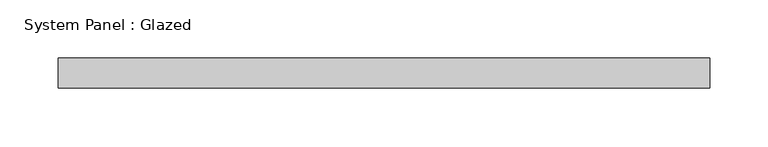
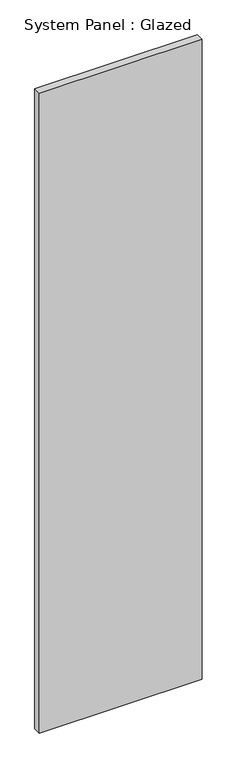
"""IFC4 building model written with IfcOpenShell, lengths in millimetres: plate geometry, System Panel : Glazed."""

from ifc_helpers import new_model, si_unit, origin, origin_with_axes, place, context, project, spatial, polyline, outline, extrude, source, transform, mapped, element, save


def system_panel_glazed_2536b6f7(model_context):
    return source(origin(), model_context, "Body", "SweptSolid", [
        extrude(outline(polyline([(278.3416667, 19.05), (-278.3416667, 19.05), (-278.3416667, 44.45), (278.3416667, 44.45), (278.3416667, 19.05)])), origin_with_axes(), (0.0, 0.0, 1.0), 2311.4),
    ])


if __name__ == "__main__":
    model = new_model("IFC4")
    model_context = context("Model", 3, world=origin())
    ifc_project = project(units=[si_unit("LENGTHUNIT", "METRE", prefix="MILLI")], contexts=[model_context])
    site = spatial("IfcSite", under=ifc_project)
    building = spatial("IfcBuilding", under=site)
    placement = place(None, origin())
    system_panel_glazed_shape = system_panel_glazed_2536b6f7(model_context)
    element("IfcPlate", 1, ObjectType="System Panel : Glazed", at=placement, inside=building, context=model_context, shape_type="MappedRepresentation", body=[
        mapped(system_panel_glazed_shape, transform((0.0, 0.0, 0.0), x_axis=(1.0, 0.0, 0.0), y_axis=(0.0, 1.0, 0.0), z_axis=(0.0, 0.0, 1.0))),
    ])
    save(model, "model.ifc")

# Revit data of these elements
# Type "System Panel : Glazed"
#   Construction Type Id = "GSP4R"
#   Analytic Construction = "1/8 in Pilkington single glazing"
#   Visual Light Transmittance = 0.9
#   Solar Heat Gain Coefficient = 0.86
#   Heat Transfer Coefficient (U) = 1.18115 BTU/(h·ft²·°F)
#   Define Thermal Properties by = 1
# Element 1 (IfcPlate, "System Panel : Glazed")
#   Materials on its faces: "Glass"
# Materials
#   "Glass": class "Glass", colour RGB 0 128 192, transparency 0.75, Description = "Soda Lime Glass", Cost = 0
